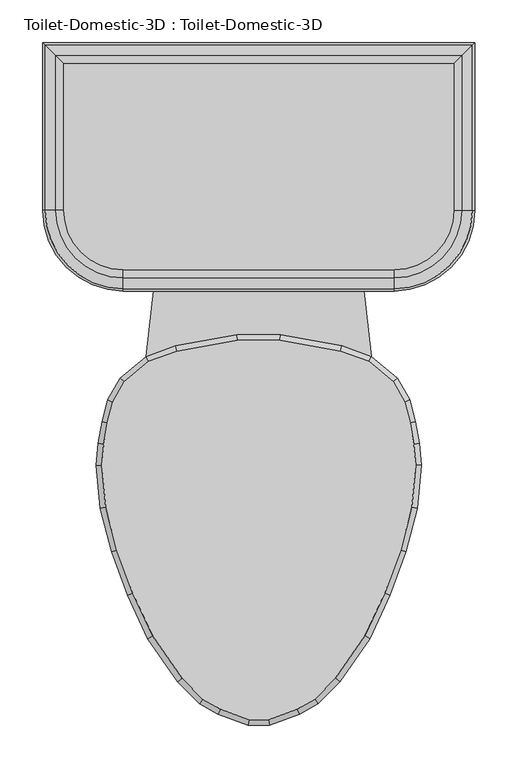
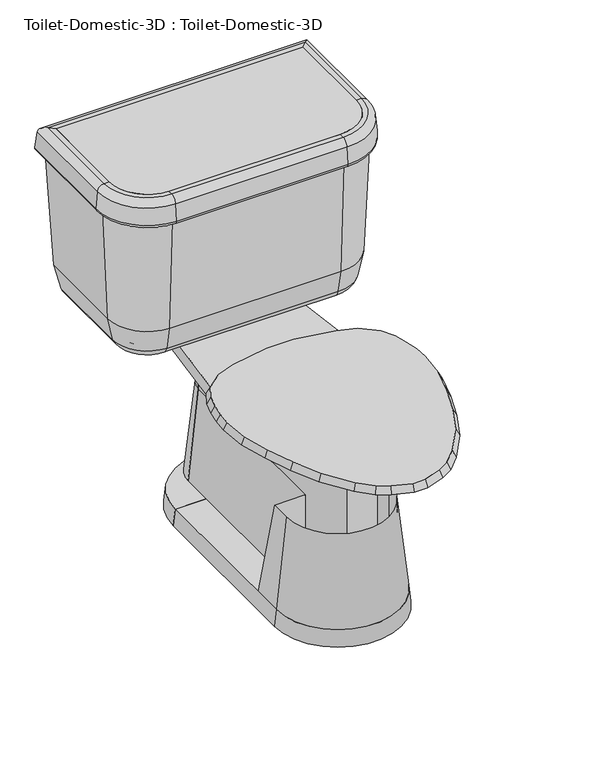
"""IFC4 building model written with IfcOpenShell, lengths in millimetres: flow terminal geometry, Toilet-Domestic-3D : Toilet-Domestic-3D."""

from ifc_helpers import new_model, si_unit, point, frame, frame_2d, origin, place, context, project, spatial, polyline, circle_curve, ellipse_curve, trimmed, segment, composite_curve, outline, extrude, faceted_brep, source, transform, mapped, element, save
from ifc_brep_helpers import plane_surface, cylinder_surface, revolved_surface, advanced_brep


def toilet_domestic_3d_toilet_domestic_3d_f7549cf7(model_context):
    return source(origin(), model_context, "Body", "SolidModel", [
        advanced_brep(
        [(-117.7636364, 285.75, 0.0), (-38.1, 285.75, 0.0), (-38.1, 285.75, 31.75), (-114.3, 285.75, 31.75), (117.7636364, 285.75, 0.0), (114.3, 285.75, 31.75), (38.1, 285.75, 31.75), (38.1, 285.75, 0.0)],
        [
            (0, 1),
            (1, 2),
            (2, 3),
            (3, 0),
            (4, 5),
            (5, 6),
            (6, 7),
            (7, 4),
            (7, 1, circle_curve(frame((0.0, 285.75, 0.0), z_axis=(0.0, 0.0, 1.0), x_axis=(-1.0, 0.0, 0.0)), 38.1)),
            (0, 4, circle_curve(frame((0.0, 285.75, 0.0), z_axis=(0.0, 0.0, -1.0), x_axis=(-1.0, 0.0, 0.0)), 117.7636364)),
            (6, 2, circle_curve(frame((0.0, 285.75, 31.75), z_axis=(0.0, 0.0, 1.0), x_axis=(-1.0, 0.0, 0.0)), 38.1)),
            (5, 3, circle_curve(frame((0.0, 285.75, 31.75), z_axis=(0.0, 0.0, 1.0), x_axis=(-1.0, 0.0, 0.0)), 114.3)),
        ],
        [
            plane_surface(frame((0.0, 285.75, -304.8), z_axis=(0.0, -1.0, 0.0), x_axis=(-1.0, 0.0, 0.0))),
            plane_surface(frame((0.0, 285.75, -304.8), z_axis=(0.0, -1.0, 0.0), x_axis=(1.0, 0.0, 0.0))),
            plane_surface(frame((0.0, 285.75, 0.0), z_axis=(0.0, 0.0, -1.0), x_axis=(-1.0, 0.0, 0.0))),
            revolved_surface(polyline([(-38.1, 285.75, 0.0), (-38.1, 285.75, 31.75)]), (0.0, 285.75, -304.8), (0.0, 0.0, -1.0)),
            plane_surface(frame((0.0, 285.75, 31.75), z_axis=(0.0, 0.0, 1.0), x_axis=(-1.0, 0.0, 0.0))),
            revolved_surface(polyline([(-114.3, 285.75, 31.75), (-117.7636364, 285.75, 0.0)]), (0.0, 285.75, -304.8), (0.0, 0.0, -1.0)),
        ],
        [
            (0, [[1, 2, 3, 4]]),
            (1, [[5, 6, 7, 8]]),
            (2, [[9, -1, 10, -8]]),
            (3, [[11, -2, -9, -7]]),
            (4, [[12, -3, -11, -6]]),
            (5, [[-10, -4, -12, -5]]),
        ],
    ),
        advanced_brep(
        [(-38.1, 342.9, 206.375), (-57.15, 342.9, 31.75), (-38.1, 342.9, 31.75), (38.1, 342.9, 206.375), (38.1, 342.9, 31.75), (57.15, 342.9, 31.75)],
        [
            (0, 1),
            (1, 2),
            (2, 0),
            (3, 4),
            (4, 5),
            (5, 3),
            (5, 1, circle_curve(frame((0.0, 342.9, 31.75), z_axis=(0.0, 0.0, 1.0), x_axis=(-1.0, 0.0, 0.0)), 57.15)),
            (0, 3, circle_curve(frame((0.0, 342.9, 206.375), z_axis=(0.0, 0.0, -1.0), x_axis=(-1.0, 0.0, 0.0)), 38.1)),
            (4, 2, circle_curve(frame((0.0, 342.9, 31.75), z_axis=(0.0, 0.0, 1.0), x_axis=(-1.0, 0.0, 0.0)), 38.1)),
        ],
        [
            plane_surface(frame((0.0, 342.9, 31.75), z_axis=(0.0, -1.0, 0.0), x_axis=(-1.0, 0.0, 0.0))),
            plane_surface(frame((0.0, 342.9, 31.75), z_axis=(0.0, -1.0, 0.0), x_axis=(1.0, 0.0, 0.0))),
            revolved_surface(polyline([(-38.1, 342.9, 206.375), (-57.15, 342.9, 31.75)]), (0.0, 342.9, 31.75), (0.0, 0.0, -1.0)),
            plane_surface(frame((0.0, 342.9, 31.75), z_axis=(0.0, 0.0, -1.0), x_axis=(-1.0, 0.0, 0.0))),
            revolved_surface(polyline([(-38.1, 342.9, 31.75), (-38.1, 342.9, 206.375)]), (0.0, 342.9, 31.75), (0.0, 0.0, -1.0)),
        ],
        [
            (0, [[1, 2, 3]]),
            (1, [[4, 5, 6]]),
            (2, [[7, -1, 8, -6]]),
            (3, [[9, -2, -7, -5]]),
            (4, [[-8, -3, -9, -4]]),
        ],
    ),
        faceted_brep([(-157.6293435, 97.472128, 400.05), (-171.060664, 73.773864, 400.05), (-177.5851102, 49.4242991, 400.05), (-181.9845715, 24.4737144, 400.05), (-184.125744, 0.0, 400.05), (-179.7950716, -49.4998127, 400.05), (-166.347, -99.688699, 400.05), (-148.0469602, -149.9676451, 400.05), (-124.7045808, -200.0255393, 400.05), (-90.0971582, -249.9125941, 400.05), (-65.691017, -274.3187354, 400.05), (-44.8990862, -286.3229622, 400.05), (-11.5803237, -298.45, 400.05), (11.5803237, -298.45, 400.05), (44.8990862, -286.3229622, 400.05), (65.691017, -274.3187354, 400.05), (90.0971582, -249.9125941, 400.05), (124.7045808, -200.0255393, 400.05), (148.0469602, -149.9676451, 400.05), (166.347, -99.688699, 400.05), (179.7950716, -49.4998127, 400.05), (184.125744, 0.0, 400.05), (181.9845715, 24.4737144, 400.05), (177.5851102, 49.4242991, 400.05), (171.060664, 73.773864, 400.05), (157.6293435, 97.472128, 400.05), (129.0942628, 121.4159037, 400.05), (95.7755003, 133.5429415, 400.05), (24.844447, 146.05, 400.05), (-24.844447, 146.05, 400.05), (-95.7755003, 133.5429415, 400.05), (-129.0942628, 121.4159037, 400.05), (-162.5887836, 101.6, 387.2181453), (-132.3182423, 127.0, 387.2181453), (-97.4252791, 139.7, 387.2181453), (-25.4, 152.4, 387.2181453), (25.4, 152.4, 387.2181453), (97.4252791, 139.7, 387.2181453), (132.3182423, 127.0, 387.2181453), (162.5887836, 101.6, 387.2181453), (176.9845865, 76.2, 387.2181453), (183.790496, 50.8, 387.2181453), (188.2862441, 25.3033453, 387.2181453), (190.5, 0.0, 387.2181453), (186.0724883, -50.6066907, 387.2181453), (172.4088722, -101.6, 387.2181453), (153.9191843, -152.4, 387.2181453), (130.2307553, -203.2, 387.2181453), (94.9900085, -254.0, 387.2181453), (69.5900085, -279.4, 387.2181453), (47.5929632, -292.1, 387.2181453), (12.7, -304.8, 387.2181453), (-12.7, -304.8, 387.2181453), (-47.5929632, -292.1, 387.2181453), (-69.5900085, -279.4, 387.2181453), (-94.9900085, -254.0, 387.2181453), (-130.2307553, -203.2, 387.2181453), (-153.9191843, -152.4, 387.2181453), (-172.4088722, -101.6, 387.2181453), (-186.0724883, -50.6066907, 387.2181453), (-190.5, 0.0, 387.2181453), (-188.2862441, 25.3033453, 387.2181453), (-183.790496, 50.8, 387.2181453), (-176.9845865, 76.2, 387.2181453)], [[[0, 1, 2, 3, 4, 5, 6, 7, 8, 9, 10, 11, 12, 13, 14, 15, 16, 17, 18, 19, 20, 21, 22, 23, 24, 25, 26, 27, 28, 29, 30, 31]], [[32, 33, 34, 35, 36, 37, 38, 39, 40, 41, 42, 43, 44, 45, 46, 47, 48, 49, 50, 51, 52, 53, 54, 55, 56, 57, 58, 59, 60, 61, 62, 63]], [[32, 63, 1, 0]], [[63, 62, 2, 1]], [[62, 61, 3, 2]], [[61, 60, 4, 3]], [[60, 59, 5, 4]], [[59, 58, 6, 5]], [[58, 57, 7, 6]], [[57, 56, 8, 7]], [[56, 55, 9, 8]], [[55, 54, 10, 9]], [[54, 53, 11, 10]], [[53, 52, 12, 11]], [[52, 51, 13, 12]], [[51, 50, 14, 13]], [[50, 49, 15, 14]], [[49, 48, 16, 15]], [[48, 47, 17, 16]], [[47, 46, 18, 17]], [[46, 45, 19, 18]], [[45, 44, 20, 19]], [[44, 43, 21, 20]], [[43, 42, 22, 21]], [[42, 41, 23, 22]], [[41, 40, 24, 23]], [[40, 39, 25, 24]], [[39, 38, 26, 25]], [[38, 37, 27, 26]], [[37, 36, 28, 27]], [[36, 35, 29, 28]], [[35, 34, 30, 29]], [[34, 33, 31, 30]], [[33, 32, 0, 31]]]),
        extrude(outline(composite_curve([segment(polyline([(228.5868869, 469.8868869), (228.5868869, 298.45)]), True, "CONTINUOUS"), segment(trimmed(circle_curve(frame_2d((158.75, 298.45)), 69.8368869), [point((228.5868869, 298.45))], [point((158.75, 228.6131131))], False, "CARTESIAN"), True, "CONTINUOUS"), segment(polyline([(158.75, 228.6131131), (-158.75, 228.6131131)]), True, "CONTINUOUS"), segment(trimmed(circle_curve(frame_2d((-158.75, 298.45)), 69.8368869), [point((-158.75, 228.6131131))], [point((-228.5868869, 298.45))], False, "CARTESIAN"), True, "CONTINUOUS"), segment(polyline([(-228.5868869, 298.45), (-228.5868869, 469.8868869), (228.5868869, 469.8868869)]), True, "CONTINUOUS")], self_intersect=False)), frame((0.0, 0.0, 654.05), z_axis=(0.0, 0.0, 1.0), x_axis=(1.0, 0.0, 0.0)), (0.0, 0.0, 1.0), 50.8),
        extrude(outline(composite_curve([segment(trimmed(circle_curve(frame_2d((0.0, 342.9)), 38.1), [point((-38.1, 342.9))], [point((38.1, 342.9))], False, "CARTESIAN"), True, "CONTINUOUS"), segment(polyline([(38.1, 342.9), (-38.1, 342.9)]), True, "CONTINUOUS")], self_intersect=False)), frame((0.0, 0.0, 206.375), z_axis=(0.0, 0.0, 1.0), x_axis=(1.0, 0.0, 0.0)), (0.0, 0.0, 1.0), 130.175),
        advanced_brep(
        [(177.8, 419.1, 387.2181453), (177.8, 419.1, 374.65), (177.8, 298.45, 374.65), (177.8, 298.45, 387.2181453), (192.8020829, 434.1020829, 387.2181453), (192.8020829, 298.45, 387.2181453), (211.4650931, 452.7650931, 402.4478636), (211.4650931, 298.45, 402.4478636), (218.7732506, 460.0732506, 438.15), (218.7732506, 298.45, 438.15), (228.5868869, 469.8868869, 654.05), (228.5868869, 298.45, 654.05), (228.5868869, 469.8868869, 704.85), (228.5868869, 298.45, 704.85), (237.91817, 479.21817, 704.85), (237.91817, 298.45, 704.85), (250.5698426, 491.8698426, 693.2568779), (250.5698426, 298.45, 693.2568779), (253.3960274, 494.6960274, 660.953439), (253.3960274, 298.45, 660.953439), (247.070191, 488.370191, 654.05), (247.070191, 298.45, 654.05), (241.3, 482.6, 654.05), (241.3, 298.45, 654.05), (231.4863636, 472.7863636, 438.15), (231.4863636, 298.45, 438.15), (222.3416824, 463.6416824, 393.4759963), (222.3416824, 298.45, 393.4759963), (197.8071664, 439.1071664, 374.65), (197.8071664, 298.45, 374.65), (158.75, 279.4, 387.2181453), (158.75, 279.4, 374.65), (158.75, 264.3979171, 387.2181453), (158.75, 245.7349069, 402.4478636), (158.75, 238.4267494, 438.15), (158.75, 228.6131131, 654.05), (158.75, 228.6131131, 704.85), (158.75, 219.28183, 704.85), (158.75, 206.6301574, 693.2568779), (158.75, 203.8039726, 660.953439), (158.75, 210.129809, 654.05), (158.75, 215.9, 654.05), (158.75, 225.7136364, 438.15), (158.75, 234.8583176, 393.4759963), (158.75, 259.3928336, 374.65), (-158.75, 279.4, 374.65), (-158.75, 279.4, 387.2181453), (-158.75, 264.3979171, 387.2181453), (-158.75, 245.7349069, 402.4478636), (-158.75, 238.4267494, 438.15), (-158.75, 228.6131131, 654.05), (-158.75, 228.6131131, 704.85), (-158.75, 219.28183, 704.85), (-158.75, 206.6301574, 693.2568779), (-158.75, 203.8039726, 660.953439), (-158.75, 210.129809, 654.05), (-158.75, 215.9, 654.05), (-158.75, 225.7136364, 438.15), (-158.75, 234.8583176, 393.4759963), (-158.75, 259.3928336, 374.65), (-177.8, 298.45, 387.2181453), (-177.8, 298.45, 374.65), (-192.8020829, 298.45, 387.2181453), (-211.4650931, 298.45, 402.4478636), (-218.7732506, 298.45, 438.15), (-228.5868869, 298.45, 654.05), (-228.5868869, 298.45, 704.85), (-237.91817, 298.45, 704.85), (-250.5698426, 298.45, 693.2568779), (-253.3960274, 298.45, 660.953439), (-247.070191, 298.45, 654.05), (-241.3, 298.45, 654.05), (-231.4863636, 298.45, 438.15), (-222.3416824, 298.45, 393.4759963), (-197.8071664, 298.45, 374.65), (-177.8, 419.1, 374.65), (-177.8, 419.1, 387.2181453), (-192.8020829, 434.1020829, 387.2181453), (-211.4650931, 452.7650931, 402.4478636), (-218.7732506, 460.0732506, 438.15), (-228.5868869, 469.8868869, 654.05), (-228.5868869, 469.8868869, 704.85), (-237.91817, 479.21817, 704.85), (-250.5698426, 491.8698426, 693.2568779), (-253.3960274, 494.6960274, 660.953439), (-247.070191, 488.370191, 654.05), (-241.3, 482.6, 654.05), (-231.4863636, 472.7863636, 438.15), (-222.3416824, 463.6416824, 393.4759963), (-197.8071664, 439.1071664, 374.65)],
        [
            (0, 1),
            (1, 2),
            (2, 3),
            (3, 0),
            (4, 0),
            (3, 5),
            (5, 4),
            (6, 4, ellipse_curve(frame((192.8020829, 434.1020829, 406.2681453), z_axis=(-0.7071067811865451, 0.7071067811865498, 0.0), x_axis=(-0.7071067811865497, -0.7071067811865452, 0.0)), 26.9407684, 19.05)),
            (5, 7, circle_curve(frame((192.8020829, 298.45, 406.2681453), z_axis=(0.0, -1.0, 0.0), x_axis=(1.0, 0.0, 0.0)), 19.05)),
            (7, 6),
            (8, 6),
            (7, 9),
            (9, 8),
            (10, 8),
            (9, 11),
            (11, 10),
            (12, 10),
            (11, 13),
            (13, 12),
            (14, 12),
            (13, 15),
            (15, 14),
            (16, 14, ellipse_curve(frame((237.91817, 479.21817, 692.15), z_axis=(0.7071067811865451, -0.7071067811865498, 0.0), x_axis=(0.7071067811865497, 0.7071067811865452, 0.0)), 17.9605122, 12.7)),
            (15, 17, circle_curve(frame((237.91817, 298.45, 692.15), z_axis=(0.0, 1.0, 0.0), x_axis=(1.0, 0.0, 0.0)), 12.7)),
            (17, 16),
            (18, 16),
            (17, 19),
            (19, 18),
            (20, 18, ellipse_curve(frame((247.070191, 488.370191, 660.4), z_axis=(0.7071067811865451, -0.7071067811865498, 0.0), x_axis=(0.7071067811865497, 0.7071067811865452, 0.0)), 8.9802561, 6.35)),
            (19, 21, circle_curve(frame((247.070191, 298.45, 660.4), z_axis=(0.0, 1.0, 0.0), x_axis=(1.0, 0.0, 0.0)), 6.35)),
            (21, 20),
            (22, 20),
            (21, 23),
            (23, 22),
            (24, 22),
            (23, 25),
            (25, 24),
            (26, 24),
            (25, 27),
            (27, 26),
            (28, 26, ellipse_curve(frame((197.8071664, 439.1071664, 400.05), z_axis=(0.7071067811865451, -0.7071067811865498, 0.0), x_axis=(0.7071067811865497, 0.7071067811865452, 0.0)), 35.9210245, 25.4)),
            (27, 29, circle_curve(frame((197.8071664, 298.45, 400.05), z_axis=(0.0, 1.0, 0.0), x_axis=(1.0, 0.0, 0.0)), 25.4)),
            (29, 28),
            (1, 28),
            (29, 2),
            (30, 3, circle_curve(frame((158.75, 298.45, 387.2181453), z_axis=(0.0, 0.0, 1.0), x_axis=(1.0, 0.0, 0.0)), 19.05)),
            (2, 31, circle_curve(frame((158.75, 298.45, 374.65), z_axis=(0.0, 0.0, -1.0), x_axis=(1.0, 0.0, 0.0)), 19.05)),
            (31, 30),
            (32, 5, circle_curve(frame((158.75, 298.45, 387.2181453), z_axis=(0.0, 0.0, 1.0), x_axis=(1.0, 0.0, 0.0)), 34.0520829)),
            (30, 32),
            (33, 7, circle_curve(frame((158.75, 298.45, 402.4478636), z_axis=(0.0, 0.0, 1.0), x_axis=(1.0, 0.0, 0.0)), 52.7150931)),
            (32, 33, circle_curve(frame((158.75, 264.3979171, 406.2681453), z_axis=(-1.0, 0.0, 0.0), x_axis=(0.0, -1.0, 0.0)), 19.05)),
            (34, 9, circle_curve(frame((158.75, 298.45, 438.15), z_axis=(0.0, 0.0, 1.0), x_axis=(1.0, 0.0, 0.0)), 60.0232506)),
            (33, 34),
            (35, 11, circle_curve(frame((158.75, 298.45, 654.05), z_axis=(0.0, 0.0, 1.0), x_axis=(1.0, 0.0, 0.0)), 69.8368869)),
            (34, 35),
            (36, 13, circle_curve(frame((158.75, 298.45, 704.85), z_axis=(0.0, 0.0, 1.0), x_axis=(1.0, 0.0, 0.0)), 69.8368869)),
            (35, 36),
            (37, 15, circle_curve(frame((158.75, 298.45, 704.85), z_axis=(0.0, 0.0, 1.0), x_axis=(1.0, 0.0, 0.0)), 79.16817)),
            (36, 37),
            (38, 17, circle_curve(frame((158.75, 298.45, 693.2568779), z_axis=(0.0, 0.0, 1.0), x_axis=(1.0, 0.0, 0.0)), 91.8198426)),
            (37, 38, circle_curve(frame((158.75, 219.28183, 692.15), z_axis=(1.0, 0.0, 0.0), x_axis=(0.0, -1.0, 0.0)), 12.7)),
            (39, 19, circle_curve(frame((158.75, 298.45, 660.953439), z_axis=(0.0, 0.0, 1.0), x_axis=(1.0, 0.0, 0.0)), 94.6460274)),
            (38, 39),
            (40, 21, circle_curve(frame((158.75, 298.45, 654.05), z_axis=(0.0, 0.0, 1.0), x_axis=(1.0, 0.0, 0.0)), 88.320191)),
            (39, 40, circle_curve(frame((158.75, 210.129809, 660.4), z_axis=(1.0, 0.0, 0.0), x_axis=(0.0, -1.0, 0.0)), 6.35)),
            (41, 23, circle_curve(frame((158.75, 298.45, 654.05), z_axis=(0.0, 0.0, 1.0), x_axis=(1.0, 0.0, 0.0)), 82.55)),
            (40, 41),
            (42, 25, circle_curve(frame((158.75, 298.45, 438.15), z_axis=(0.0, 0.0, 1.0), x_axis=(1.0, 0.0, 0.0)), 72.7363636)),
            (41, 42),
            (43, 27, circle_curve(frame((158.75, 298.45, 393.4759963), z_axis=(0.0, 0.0, 1.0), x_axis=(1.0, 0.0, 0.0)), 63.5916824)),
            (42, 43),
            (44, 29, circle_curve(frame((158.75, 298.45, 374.65), z_axis=(0.0, 0.0, 1.0), x_axis=(1.0, 0.0, 0.0)), 39.0571664)),
            (43, 44, circle_curve(frame((158.75, 259.3928336, 400.05), z_axis=(1.0, 0.0, 0.0), x_axis=(0.0, -1.0, 0.0)), 25.4)),
            (44, 31),
            (31, 45),
            (45, 46),
            (46, 30),
            (46, 47),
            (47, 32),
            (47, 48, circle_curve(frame((-158.75, 264.3979171, 406.2681453), z_axis=(-1.0, 0.0, 0.0), x_axis=(0.0, -1.0, 0.0)), 19.05)),
            (48, 33),
            (48, 49),
            (49, 34),
            (49, 50),
            (50, 35),
            (50, 51),
            (51, 36),
            (51, 52),
            (52, 37),
            (52, 53, circle_curve(frame((-158.75, 219.28183, 692.15), z_axis=(1.0, 0.0, 0.0), x_axis=(0.0, -1.0, 0.0)), 12.7)),
            (53, 38),
            (53, 54),
            (54, 39),
            (54, 55, circle_curve(frame((-158.75, 210.129809, 660.4), z_axis=(1.0, 0.0, 0.0), x_axis=(0.0, -1.0, 0.0)), 6.35)),
            (55, 40),
            (55, 56),
            (56, 41),
            (56, 57),
            (57, 42),
            (57, 58),
            (58, 43),
            (58, 59, circle_curve(frame((-158.75, 259.3928336, 400.05), z_axis=(1.0, 0.0, 0.0), x_axis=(0.0, -1.0, 0.0)), 25.4)),
            (59, 44),
            (59, 45),
            (60, 46, circle_curve(frame((-158.75, 298.45, 387.2181453), z_axis=(0.0, 0.0, 1.0), x_axis=(0.0, -1.0, 0.0)), 19.05)),
            (45, 61, circle_curve(frame((-158.75, 298.45, 374.65), z_axis=(0.0, 0.0, -1.0), x_axis=(0.0, -1.0, 0.0)), 19.05)),
            (61, 60),
            (62, 47, circle_curve(frame((-158.75, 298.45, 387.2181453), z_axis=(0.0, 0.0, 1.0), x_axis=(0.0, -1.0, 0.0)), 34.0520829)),
            (60, 62),
            (63, 48, circle_curve(frame((-158.75, 298.45, 402.4478636), z_axis=(0.0, 0.0, 1.0), x_axis=(0.0, -1.0, 0.0)), 52.7150931)),
            (62, 63, circle_curve(frame((-192.8020829, 298.45, 406.2681453), z_axis=(0.0, 1.0, 0.0), x_axis=(-1.0, 0.0, 0.0)), 19.05)),
            (64, 49, circle_curve(frame((-158.75, 298.45, 438.15), z_axis=(0.0, 0.0, 1.0), x_axis=(0.0, -1.0, 0.0)), 60.0232506)),
            (63, 64),
            (65, 50, circle_curve(frame((-158.75, 298.45, 654.05), z_axis=(0.0, 0.0, 1.0), x_axis=(0.0, -1.0, 0.0)), 69.8368869)),
            (64, 65),
            (66, 51, circle_curve(frame((-158.75, 298.45, 704.85), z_axis=(0.0, 0.0, 1.0), x_axis=(0.0, -1.0, 0.0)), 69.8368869)),
            (65, 66),
            (67, 52, circle_curve(frame((-158.75, 298.45, 704.85), z_axis=(0.0, 0.0, 1.0), x_axis=(0.0, -1.0, 0.0)), 79.16817)),
            (66, 67),
            (68, 53, circle_curve(frame((-158.75, 298.45, 693.2568779), z_axis=(0.0, 0.0, 1.0), x_axis=(0.0, -1.0, 0.0)), 91.8198426)),
            (67, 68, circle_curve(frame((-237.91817, 298.45, 692.15), z_axis=(0.0, -1.0, 0.0), x_axis=(-1.0, 0.0, 0.0)), 12.7)),
            (69, 54, circle_curve(frame((-158.75, 298.45, 660.953439), z_axis=(0.0, 0.0, 1.0), x_axis=(0.0, -1.0, 0.0)), 94.6460274)),
            (68, 69),
            (70, 55, circle_curve(frame((-158.75, 298.45, 654.05), z_axis=(0.0, 0.0, 1.0), x_axis=(0.0, -1.0, 0.0)), 88.320191)),
            (69, 70, circle_curve(frame((-247.070191, 298.45, 660.4), z_axis=(0.0, -1.0, 0.0), x_axis=(-1.0, 0.0, 0.0)), 6.35)),
            (71, 56, circle_curve(frame((-158.75, 298.45, 654.05), z_axis=(0.0, 0.0, 1.0), x_axis=(0.0, -1.0, 0.0)), 82.55)),
            (70, 71),
            (72, 57, circle_curve(frame((-158.75, 298.45, 438.15), z_axis=(0.0, 0.0, 1.0), x_axis=(0.0, -1.0, 0.0)), 72.7363636)),
            (71, 72),
            (73, 58, circle_curve(frame((-158.75, 298.45, 393.4759963), z_axis=(0.0, 0.0, 1.0), x_axis=(0.0, -1.0, 0.0)), 63.5916824)),
            (72, 73),
            (74, 59, circle_curve(frame((-158.75, 298.45, 374.65), z_axis=(0.0, 0.0, 1.0), x_axis=(0.0, -1.0, 0.0)), 39.0571664)),
            (73, 74, circle_curve(frame((-197.8071664, 298.45, 400.05), z_axis=(0.0, -1.0, 0.0), x_axis=(-1.0, 0.0, 0.0)), 25.4)),
            (74, 61),
            (61, 75),
            (75, 76),
            (76, 60),
            (76, 77),
            (77, 62),
            (77, 78, ellipse_curve(frame((-192.8020829, 434.1020829, 406.2681453), z_axis=(0.7071067811865498, 0.7071067811865451, 0.0), x_axis=(-0.7071067811865451, 0.70710678118655, 0.0)), 26.9407684, 19.05)),
            (78, 63),
            (78, 79),
            (79, 64),
            (79, 80),
            (80, 65),
            (80, 81),
            (81, 66),
            (81, 82),
            (82, 67),
            (82, 83, ellipse_curve(frame((-237.91817, 479.21817, 692.15), z_axis=(-0.7071067811865498, -0.7071067811865451, 0.0), x_axis=(0.7071067811865451, -0.70710678118655, 0.0)), 17.9605122, 12.7)),
            (83, 68),
            (83, 84),
            (84, 69),
            (84, 85, ellipse_curve(frame((-247.070191, 488.370191, 660.4), z_axis=(-0.7071067811865498, -0.7071067811865451, 0.0), x_axis=(0.7071067811865451, -0.70710678118655, 0.0)), 8.9802561, 6.35)),
            (85, 70),
            (85, 86),
            (86, 71),
            (86, 87),
            (87, 72),
            (87, 88),
            (88, 73),
            (88, 89, ellipse_curve(frame((-197.8071664, 439.1071664, 400.05), z_axis=(-0.7071067811865498, -0.7071067811865451, 0.0), x_axis=(0.7071067811865451, -0.70710678118655, 0.0)), 35.9210245, 25.4)),
            (89, 74),
            (89, 75),
            (75, 1),
            (0, 76),
            (4, 77),
            (6, 78),
            (8, 79),
            (10, 80),
            (12, 81),
            (14, 82),
            (16, 83),
            (18, 84),
            (20, 85),
            (22, 86),
            (24, 87),
            (26, 88),
            (28, 89),
        ],
        [
            plane_surface(frame((177.8, 419.1, 374.65), z_axis=(-1.0, 0.0, 0.0), x_axis=(0.0, -1.0, 0.0))),
            plane_surface(frame((177.8, 419.1, 387.2181453), z_axis=(0.0, 0.0, 1.0), x_axis=(0.0, -1.0, 0.0))),
            revolved_surface(polyline([(211.8520829, 298.45, 406.2681453), (211.8520829, 453.1520829260162, 406.2681453)]), (192.8020829, 419.1, 406.2681453), (0.0, -1.0, 0.0)),
            plane_surface(frame((211.4650931, 452.7650931, 402.4478636), z_axis=(-0.9796855721787505, 0.0, 0.2005397209153197), x_axis=(0.0, -1.0, 0.0))),
            plane_surface(frame((218.7732506, 460.0732506, 438.15), z_axis=(-0.9989685402102995, 0.0, 0.045407660918654086), x_axis=(0.0, -1.0, 0.0))),
            plane_surface(frame((228.5868869, 469.8868869, 654.05), z_axis=(-1.0, 0.0, 0.0), x_axis=(0.0, -1.0, 0.0))),
            plane_surface(frame((228.5868869, 469.8868869, 704.85), z_axis=(0.0, 0.0, 1.0), x_axis=(0.0, -1.0, 0.0))),
            cylinder_surface(frame((237.91817, 419.1, 692.15), z_axis=(0.0, 1.0, 0.0), x_axis=(1.0, 0.0, 0.0)), 12.7),
            plane_surface(frame((250.5698426, 491.8698426, 693.2568779), z_axis=(0.9961946980917452, 0.0, 0.08715574274766269), x_axis=(0.0, -1.0, 0.0))),
            cylinder_surface(frame((247.070191, 419.1, 660.4), z_axis=(0.0, 1.0, 0.0), x_axis=(1.0, 0.0, 0.0)), 6.35),
            plane_surface(frame((247.070191, 488.370191, 654.05), z_axis=(0.0, 0.0, -1.0), x_axis=(0.0, -1.0, 0.0))),
            plane_surface(frame((241.3, 482.6, 654.05), z_axis=(0.9989685402102993, 0.0, -0.04540766091865594), x_axis=(0.0, -1.0, 0.0))),
            plane_surface(frame((231.4863636, 472.7863636, 438.15), z_axis=(0.9796855721787489, 0.0, -0.20053972091532798), x_axis=(0.0, -1.0, 0.0))),
            cylinder_surface(frame((197.8071664, 419.1, 400.05), z_axis=(0.0, 1.0, 0.0), x_axis=(1.0, 0.0, 0.0)), 25.4),
            plane_surface(frame((197.8071664, 439.1071664, 374.65), z_axis=(0.0, 0.0, -1.0), x_axis=(0.0, -1.0, 0.0))),
            revolved_surface(polyline([(177.8, 298.45, 374.65), (177.8, 298.45, 387.2181453)]), (158.75, 298.45, 0.0), (0.0, 0.0, -1.0)),
            plane_surface(frame((158.75, 298.45, 387.2181453), z_axis=(0.0, 0.0, 1.0), x_axis=(1.0, 0.0, 0.0))),
            revolved_surface(trimmed(ellipse_curve(frame((192.8020829, 298.45, 406.2681453), z_axis=(0.0, -1.0, 0.0), x_axis=(1.0, 0.0, 0.0)), 19.05, 19.05), [point((192.8020829, 298.45, 387.2181453))], [point((211.4650931, 298.45, 402.4478636))], True, "CARTESIAN"), (158.75, 298.45, 0.0), (0.0, 0.0, -1.0)),
            revolved_surface(polyline([(211.4650931, 298.45, 402.4478636), (218.7732506, 298.45, 438.15)]), (158.75, 298.45, 0.0), (0.0, 0.0, -1.0)),
            revolved_surface(polyline([(218.7732506, 298.45, 438.15), (228.5868869, 298.45, 654.05)]), (158.75, 298.45, 0.0), (0.0, 0.0, -1.0)),
            revolved_surface(polyline([(228.5868869, 298.45, 654.05), (228.5868869, 298.45, 704.85)]), (158.75, 298.45, 0.0), (0.0, 0.0, -1.0)),
            plane_surface(frame((158.75, 298.45, 704.85), z_axis=(0.0, 0.0, 1.0), x_axis=(1.0, 0.0, 0.0))),
            revolved_surface(trimmed(ellipse_curve(frame((237.91817, 298.45, 692.15), z_axis=(0.0, 1.0, 0.0), x_axis=(1.0, 0.0, 0.0)), 12.7, 12.7), [point((237.91817, 298.45, 704.85))], [point((250.5698426, 298.45, 693.2568779))], True, "CARTESIAN"), (158.75, 298.45, 0.0), (0.0, 0.0, -1.0)),
            revolved_surface(polyline([(250.5698426, 298.45, 693.2568779), (253.3960274, 298.45, 660.953439)]), (158.75, 298.45, 0.0), (0.0, 0.0, -1.0)),
            revolved_surface(trimmed(ellipse_curve(frame((247.070191, 298.45, 660.4), z_axis=(0.0, 1.0, 0.0), x_axis=(1.0, 0.0, 0.0)), 6.35, 6.35), [point((253.3960274, 298.45, 660.953439))], [point((247.070191, 298.45, 654.05))], True, "CARTESIAN"), (158.75, 298.45, 0.0), (0.0, 0.0, -1.0)),
            plane_surface(frame((158.75, 298.45, 654.05), z_axis=(0.0, 0.0, -1.0), x_axis=(1.0, 0.0, 0.0))),
            revolved_surface(polyline([(241.3, 298.45, 654.05), (231.4863636, 298.45, 438.15)]), (158.75, 298.45, 0.0), (0.0, 0.0, -1.0)),
            revolved_surface(polyline([(231.4863636, 298.45, 438.15), (222.3416824, 298.45, 393.4759963)]), (158.75, 298.45, 0.0), (0.0, 0.0, -1.0)),
            revolved_surface(trimmed(ellipse_curve(frame((197.8071664, 298.45, 400.05), z_axis=(0.0, 1.0, 0.0), x_axis=(1.0, 0.0, 0.0)), 25.4, 25.4), [point((222.3416824, 298.45, 393.4759963))], [point((197.8071664, 298.45, 374.65))], True, "CARTESIAN"), (158.75, 298.45, 0.0), (0.0, 0.0, -1.0)),
            plane_surface(frame((158.75, 298.45, 374.65), z_axis=(0.0, 0.0, -1.0), x_axis=(1.0, 0.0, 0.0))),
            plane_surface(frame((158.75, 279.4, 374.65), z_axis=(0.0, 1.0, 0.0), x_axis=(-1.0, 0.0, 0.0))),
            plane_surface(frame((158.75, 279.4, 387.2181453), z_axis=(0.0, 0.0, 1.0), x_axis=(-1.0, 0.0, 0.0))),
            revolved_surface(polyline([(-158.75, 245.34791709999996, 406.2681453), (158.75, 245.34791709999996, 406.2681453)]), (158.75, 264.3979171, 406.2681453), (-1.0, 0.0, 0.0)),
            plane_surface(frame((158.75, 245.7349069, 402.4478636), z_axis=(0.0, 0.9796855721787505, 0.2005397209153197), x_axis=(-1.0, 0.0, 0.0))),
            plane_surface(frame((158.75, 238.4267494, 438.15), z_axis=(0.0, 0.9989685402102995, 0.045407660918654086), x_axis=(-1.0, 0.0, 0.0))),
            plane_surface(frame((158.75, 228.6131131, 654.05), z_axis=(0.0, 1.0, 0.0), x_axis=(-1.0, 0.0, 0.0))),
            plane_surface(frame((158.75, 228.6131131, 704.85), z_axis=(0.0, 0.0, 1.0), x_axis=(-1.0, 0.0, 0.0))),
            cylinder_surface(frame((158.75, 219.28183, 692.15), z_axis=(1.0, 0.0, 0.0), x_axis=(0.0, -1.0, 0.0)), 12.7),
            plane_surface(frame((158.75, 206.6301574, 693.2568779), z_axis=(0.0, -0.9961946980917452, 0.08715574274766269), x_axis=(-1.0, 0.0, 0.0))),
            cylinder_surface(frame((158.75, 210.129809, 660.4), z_axis=(1.0, 0.0, 0.0), x_axis=(0.0, -1.0, 0.0)), 6.35),
            plane_surface(frame((158.75, 210.129809, 654.05), z_axis=(0.0, 0.0, -1.0), x_axis=(-1.0, 0.0, 0.0))),
            plane_surface(frame((158.75, 215.9, 654.05), z_axis=(0.0, -0.9989685402102993, -0.04540766091865594), x_axis=(-1.0, 0.0, 0.0))),
            plane_surface(frame((158.75, 225.7136364, 438.15), z_axis=(0.0, -0.9796855721787489, -0.20053972091532798), x_axis=(-1.0, 0.0, 0.0))),
            cylinder_surface(frame((158.75, 259.3928336, 400.05), z_axis=(1.0, 0.0, 0.0), x_axis=(0.0, -1.0, 0.0)), 25.4),
            plane_surface(frame((158.75, 259.3928336, 374.65), z_axis=(0.0, 0.0, -1.0), x_axis=(-1.0, 0.0, 0.0))),
            revolved_surface(polyline([(-158.75, 279.4, 374.65), (-158.75, 279.4, 387.2181453)]), (-158.75, 298.45, 0.0), (0.0, 0.0, -1.0)),
            plane_surface(frame((-158.75, 298.45, 387.2181453), z_axis=(0.0, 0.0, 1.0), x_axis=(0.0, -1.0, 0.0))),
            revolved_surface(trimmed(ellipse_curve(frame((-158.75, 264.3979171, 406.2681453), z_axis=(-1.0, 0.0, 0.0), x_axis=(0.0, -1.0, 0.0)), 19.05, 19.05), [point((-158.75, 264.3979171, 387.2181453))], [point((-158.75, 245.7349069, 402.4478636))], True, "CARTESIAN"), (-158.75, 298.45, 0.0), (0.0, 0.0, -1.0)),
            revolved_surface(polyline([(-158.75, 245.7349069, 402.4478636), (-158.75, 238.4267494, 438.15)]), (-158.75, 298.45, 0.0), (0.0, 0.0, -1.0)),
            revolved_surface(polyline([(-158.75, 238.4267494, 438.15), (-158.75, 228.6131131, 654.05)]), (-158.75, 298.45, 0.0), (0.0, 0.0, -1.0)),
            revolved_surface(polyline([(-158.75, 228.6131131, 654.05), (-158.75, 228.6131131, 704.85)]), (-158.75, 298.45, 0.0), (0.0, 0.0, -1.0)),
            plane_surface(frame((-158.75, 298.45, 704.85), z_axis=(0.0, 0.0, 1.0), x_axis=(0.0, -1.0, 0.0))),
            revolved_surface(trimmed(ellipse_curve(frame((-158.75, 219.28183, 692.15), z_axis=(1.0, 0.0, 0.0), x_axis=(0.0, -1.0, 0.0)), 12.7, 12.7), [point((-158.75, 219.28183, 704.85))], [point((-158.75, 206.6301574, 693.2568779))], True, "CARTESIAN"), (-158.75, 298.45, 0.0), (0.0, 0.0, -1.0)),
            revolved_surface(polyline([(-158.75, 206.6301574, 693.2568779), (-158.75, 203.8039726, 660.953439)]), (-158.75, 298.45, 0.0), (0.0, 0.0, -1.0)),
            revolved_surface(trimmed(ellipse_curve(frame((-158.75, 210.129809, 660.4), z_axis=(1.0, 0.0, 0.0), x_axis=(0.0, -1.0, 0.0)), 6.35, 6.35), [point((-158.75, 203.8039726, 660.953439))], [point((-158.75, 210.129809, 654.05))], True, "CARTESIAN"), (-158.75, 298.45, 0.0), (0.0, 0.0, -1.0)),
            plane_surface(frame((-158.75, 298.45, 654.05), z_axis=(0.0, 0.0, -1.0), x_axis=(0.0, -1.0, 0.0))),
            revolved_surface(polyline([(-158.75, 215.9, 654.05), (-158.75, 225.7136364, 438.15)]), (-158.75, 298.45, 0.0), (0.0, 0.0, -1.0)),
            revolved_surface(polyline([(-158.75, 225.7136364, 438.15), (-158.75, 234.8583176, 393.4759963)]), (-158.75, 298.45, 0.0), (0.0, 0.0, -1.0)),
            revolved_surface(trimmed(ellipse_curve(frame((-158.75, 259.3928336, 400.05), z_axis=(1.0, 0.0, 0.0), x_axis=(0.0, -1.0, 0.0)), 25.4, 25.4), [point((-158.75, 234.8583176, 393.4759963))], [point((-158.75, 259.3928336, 374.65))], True, "CARTESIAN"), (-158.75, 298.45, 0.0), (0.0, 0.0, -1.0)),
            plane_surface(frame((-158.75, 298.45, 374.65), z_axis=(0.0, 0.0, -1.0), x_axis=(0.0, -1.0, 0.0))),
            plane_surface(frame((-177.8, 298.45, 374.65), z_axis=(1.0, 0.0, 0.0), x_axis=(0.0, 1.0, 0.0))),
            plane_surface(frame((-177.8, 298.45, 387.2181453), z_axis=(0.0, 0.0, 1.0), x_axis=(0.0, 1.0, 0.0))),
            revolved_surface(polyline([(-211.8520829, 453.15208292601636, 406.2681453), (-211.8520829, 298.45, 406.2681453)]), (-192.8020829, 298.45, 406.2681453), (0.0, 1.0, 0.0)),
            plane_surface(frame((-211.4650931, 298.45, 402.4478636), z_axis=(0.9796855721787505, 0.0, 0.2005397209153197), x_axis=(0.0, 1.0, 0.0))),
            plane_surface(frame((-218.7732506, 298.45, 438.15), z_axis=(0.9989685402102995, 0.0, 0.045407660918654086), x_axis=(0.0, 1.0, 0.0))),
            plane_surface(frame((-228.5868869, 298.45, 654.05), z_axis=(1.0, 0.0, 0.0), x_axis=(0.0, 1.0, 0.0))),
            plane_surface(frame((-228.5868869, 298.45, 704.85), z_axis=(0.0, 0.0, 1.0), x_axis=(0.0, 1.0, 0.0))),
            cylinder_surface(frame((-237.91817, 298.45, 692.15), z_axis=(0.0, -1.0, 0.0), x_axis=(-1.0, 0.0, 0.0)), 12.7),
            plane_surface(frame((-250.5698426, 298.45, 693.2568779), z_axis=(-0.9961946980917452, 0.0, 0.08715574274766269), x_axis=(0.0, 1.0, 0.0))),
            cylinder_surface(frame((-247.070191, 298.45, 660.4), z_axis=(0.0, -1.0, 0.0), x_axis=(-1.0, 0.0, 0.0)), 6.35),
            plane_surface(frame((-247.070191, 298.45, 654.05), z_axis=(0.0, 0.0, -1.0), x_axis=(0.0, 1.0, 0.0))),
            plane_surface(frame((-241.3, 298.45, 654.05), z_axis=(-0.9989685402102993, 0.0, -0.04540766091865594), x_axis=(0.0, 1.0, 0.0))),
            plane_surface(frame((-231.4863636, 298.45, 438.15), z_axis=(-0.9796855721787489, 0.0, -0.20053972091532798), x_axis=(0.0, 1.0, 0.0))),
            cylinder_surface(frame((-197.8071664, 298.45, 400.05), z_axis=(0.0, -1.0, 0.0), x_axis=(-1.0, 0.0, 0.0)), 25.4),
            plane_surface(frame((-197.8071664, 298.45, 374.65), z_axis=(0.0, 0.0, -1.0), x_axis=(0.0, 1.0, 0.0))),
            plane_surface(frame((-177.8, 419.1, 374.65), z_axis=(0.0, -1.0, 0.0), x_axis=(1.0, 0.0, 0.0))),
            plane_surface(frame((-177.8, 419.1, 387.2181453), z_axis=(0.0, 0.0, 1.0), x_axis=(1.0, 0.0, 0.0))),
            revolved_surface(polyline([(211.85208292601635, 453.15208290000004, 406.2681453), (-211.85208292601618, 453.15208290000004, 406.2681453)]), (-177.8, 434.1020829, 406.2681453), (1.0, 0.0, 0.0)),
            plane_surface(frame((-211.4650931, 452.7650931, 402.4478636), z_axis=(0.0, -0.9796855721787505, 0.2005397209153197), x_axis=(1.0, 0.0, 0.0))),
            plane_surface(frame((-218.7732506, 460.0732506, 438.15), z_axis=(0.0, -0.9989685402102995, 0.045407660918654086), x_axis=(1.0, 0.0, 0.0))),
            plane_surface(frame((-228.5868869, 469.8868869, 654.05), z_axis=(0.0, -1.0, 0.0), x_axis=(1.0, 0.0, 0.0))),
            plane_surface(frame((-228.5868869, 469.8868869, 704.85), z_axis=(0.0, 0.0, 1.0), x_axis=(1.0, 0.0, 0.0))),
            cylinder_surface(frame((-177.8, 479.21817, 692.15), z_axis=(-1.0, 0.0, 0.0), x_axis=(0.0, 1.0, 0.0)), 12.7),
            plane_surface(frame((-250.5698426, 491.8698426, 693.2568779), z_axis=(0.0, 0.9961946980917452, 0.08715574274766269), x_axis=(1.0, 0.0, 0.0))),
            cylinder_surface(frame((-177.8, 488.370191, 660.4), z_axis=(-1.0, 0.0, 0.0), x_axis=(0.0, 1.0, 0.0)), 6.35),
            plane_surface(frame((-247.070191, 488.370191, 654.05), z_axis=(0.0, 0.0, -1.0), x_axis=(1.0, 0.0, 0.0))),
            plane_surface(frame((-241.3, 482.6, 654.05), z_axis=(0.0, 0.9989685402102993, -0.04540766091865594), x_axis=(1.0, 0.0, 0.0))),
            plane_surface(frame((-231.4863636, 472.7863636, 438.15), z_axis=(0.0, 0.9796855721787489, -0.20053972091532798), x_axis=(1.0, 0.0, 0.0))),
            cylinder_surface(frame((-177.8, 439.1071664, 400.05), z_axis=(-1.0, 0.0, 0.0), x_axis=(0.0, 1.0, 0.0)), 25.4),
            plane_surface(frame((-197.8071664, 439.1071664, 374.65), z_axis=(0.0, 0.0, -1.0), x_axis=(1.0, 0.0, 0.0))),
        ],
        [
            (0, [[1, 2, 3, 4]]),
            (1, [[5, -4, 6, 7]]),
            (2, [[8, -7, 9, 10]]),
            (3, [[11, -10, 12, 13]]),
            (4, [[14, -13, 15, 16]]),
            (5, [[17, -16, 18, 19]]),
            (6, [[20, -19, 21, 22]]),
            (7, [[23, -22, 24, 25]]),
            (8, [[26, -25, 27, 28]]),
            (9, [[29, -28, 30, 31]]),
            (10, [[32, -31, 33, 34]]),
            (11, [[35, -34, 36, 37]]),
            (12, [[38, -37, 39, 40]]),
            (13, [[41, -40, 42, 43]]),
            (14, [[44, -43, 45, -2]]),
            (15, [[46, -3, 47, 48]]),
            (16, [[49, -6, -46, 50]]),
            (17, [[51, -9, -49, 52]]),
            (18, [[53, -12, -51, 54]]),
            (19, [[55, -15, -53, 56]]),
            (20, [[57, -18, -55, 58]]),
            (21, [[59, -21, -57, 60]]),
            (22, [[61, -24, -59, 62]]),
            (23, [[63, -27, -61, 64]]),
            (24, [[65, -30, -63, 66]]),
            (25, [[67, -33, -65, 68]]),
            (26, [[69, -36, -67, 70]]),
            (27, [[71, -39, -69, 72]]),
            (28, [[73, -42, -71, 74]]),
            (29, [[-47, -45, -73, 75]]),
            (30, [[-48, 76, 77, 78]]),
            (31, [[-50, -78, 79, 80]]),
            (32, [[-52, -80, 81, 82]]),
            (33, [[-54, -82, 83, 84]]),
            (34, [[-56, -84, 85, 86]]),
            (35, [[-58, -86, 87, 88]]),
            (36, [[-60, -88, 89, 90]]),
            (37, [[-62, -90, 91, 92]]),
            (38, [[-64, -92, 93, 94]]),
            (39, [[-66, -94, 95, 96]]),
            (40, [[-68, -96, 97, 98]]),
            (41, [[-70, -98, 99, 100]]),
            (42, [[-72, -100, 101, 102]]),
            (43, [[-74, -102, 103, 104]]),
            (44, [[-75, -104, 105, -76]]),
            (45, [[106, -77, 107, 108]]),
            (46, [[109, -79, -106, 110]]),
            (47, [[111, -81, -109, 112]]),
            (48, [[113, -83, -111, 114]]),
            (49, [[115, -85, -113, 116]]),
            (50, [[117, -87, -115, 118]]),
            (51, [[119, -89, -117, 120]]),
            (52, [[121, -91, -119, 122]]),
            (53, [[123, -93, -121, 124]]),
            (54, [[125, -95, -123, 126]]),
            (55, [[127, -97, -125, 128]]),
            (56, [[129, -99, -127, 130]]),
            (57, [[131, -101, -129, 132]]),
            (58, [[133, -103, -131, 134]]),
            (59, [[-107, -105, -133, 135]]),
            (60, [[-108, 136, 137, 138]]),
            (61, [[-110, -138, 139, 140]]),
            (62, [[-112, -140, 141, 142]]),
            (63, [[-114, -142, 143, 144]]),
            (64, [[-116, -144, 145, 146]]),
            (65, [[-118, -146, 147, 148]]),
            (66, [[-120, -148, 149, 150]]),
            (67, [[-122, -150, 151, 152]]),
            (68, [[-124, -152, 153, 154]]),
            (69, [[-126, -154, 155, 156]]),
            (70, [[-128, -156, 157, 158]]),
            (71, [[-130, -158, 159, 160]]),
            (72, [[-132, -160, 161, 162]]),
            (73, [[-134, -162, 163, 164]]),
            (74, [[-135, -164, 165, -136]]),
            (75, [[-137, 166, -1, 167]]),
            (76, [[-139, -167, -5, 168]]),
            (77, [[-141, -168, -8, 169]]),
            (78, [[-143, -169, -11, 170]]),
            (79, [[-145, -170, -14, 171]]),
            (80, [[-147, -171, -17, 172]]),
            (81, [[-149, -172, -20, 173]]),
            (82, [[-151, -173, -23, 174]]),
            (83, [[-153, -174, -26, 175]]),
            (84, [[-155, -175, -29, 176]]),
            (85, [[-157, -176, -32, 177]]),
            (86, [[-159, -177, -35, 178]]),
            (87, [[-161, -178, -38, 179]]),
            (88, [[-163, -179, -41, 180]]),
            (89, [[-165, -180, -44, -166]]),
        ],
    ),
        extrude(outline(composite_curve([segment(polyline([(-25.4, 152.4), (-97.4252791, 139.7), (-132.3182423, 127.0), (-101.4824733, 395.1508638)]), True, "CONTINUOUS"), segment(trimmed(circle_curve(frame_2d((-88.8656197, 393.7)), 12.7), [point((-101.4824733, 395.1508638))], [point((-88.8656197, 406.4))], False, "CARTESIAN"), True, "CONTINUOUS"), segment(polyline([(-88.8656197, 406.4), (88.8656197, 406.4)]), True, "CONTINUOUS"), segment(trimmed(circle_curve(frame_2d((88.8656197, 393.7)), 12.7), [point((88.8656197, 406.4))], [point((101.4824733, 395.1508638))], False, "CARTESIAN"), True, "CONTINUOUS"), segment(polyline([(101.4824733, 395.1508638), (132.3182423, 127.0), (97.4252791, 139.7), (25.4, 152.4), (0.0, 152.4), (-25.4, 152.4)]), True, "CONTINUOUS")], self_intersect=False)), frame((0.0, 0.0, 336.55), z_axis=(0.0, 0.0, 1.0), x_axis=(1.0, 0.0, 0.0)), (0.0, 0.0, 1.0), 25.4),
        extrude(outline(polyline([(139.7, 264.5247209), (152.4, 336.55), (342.9, 336.55), (342.9, 206.375), (107.4852632, 206.375), (127.0, 229.6317577), (139.7, 264.5247209)])), frame((-38.1, 0.0, 0.0), z_axis=(1.0, 0.0, 0.0), x_axis=(0.0, 1.0, 0.0)), (0.0, 0.0, 1.0), 76.2),
        advanced_brep(
        [(-117.7636364, 285.75, 0.0), (-114.3, 285.75, 31.75), (-38.1, 285.75, 31.75), (-38.1, 285.75, 0.0), (-117.7636364, -38.0999951, 0.0), (-114.3, -38.0999951, 31.75), (-38.1, -38.0999951, 31.75), (-38.1, -38.0999951, 0.0), (114.2999707, -38.0999951, 31.75), (117.7636071, -38.0999951, 0.0), (38.0999707, -38.0999951, 31.75), (38.0999707, -38.0999951, 0.0), (117.7636071, 285.6681634, 0.0), (38.0999707, 285.6681634, 0.0), (38.0999707, 285.6681634, 31.75), (114.2999707, 285.6681634, 31.75)],
        [
            (0, 1),
            (1, 2),
            (2, 3),
            (3, 0),
            (0, 4),
            (4, 5),
            (5, 1),
            (5, 6),
            (6, 2),
            (6, 7),
            (7, 3),
            (7, 4),
            (8, 5, circle_curve(frame((-1.46e-05, -38.0999951, 31.75), z_axis=(0.0, 0.0, -1.0), x_axis=(-1.0, 0.0, 0.0)), 114.2999854)),
            (4, 9, circle_curve(frame((-1.46e-05, -38.0999951, 0.0), z_axis=(0.0, 0.0, 1.0), x_axis=(-1.0, 0.0, 0.0)), 117.7636217)),
            (9, 8),
            (10, 6, circle_curve(frame((-1.46e-05, -38.0999951, 31.75), z_axis=(0.0, 0.0, -1.0), x_axis=(-1.0, 0.0, 0.0)), 38.0999854)),
            (8, 10),
            (11, 7, circle_curve(frame((-1.46e-05, -38.0999951, 0.0), z_axis=(0.0, 0.0, -1.0), x_axis=(-1.0, 0.0, 0.0)), 38.0999854)),
            (10, 11),
            (11, 9),
            (12, 13),
            (13, 14),
            (14, 15),
            (15, 12),
            (9, 12),
            (15, 8),
            (14, 10),
            (13, 11),
        ],
        [
            plane_surface(frame((-196.85, 285.75, 0.0), z_axis=(0.0, 1.0, 0.0), x_axis=(0.0, 0.0, -1.0))),
            plane_surface(frame((-117.7636364, 285.75, 0.0), z_axis=(-0.9941021766079929, 0.0, 0.10844751017543448), x_axis=(0.0, -1.0, 0.0))),
            plane_surface(frame((-114.3, 285.75, 31.75), z_axis=(0.0, 0.0, 1.0), x_axis=(0.0, -1.0, 0.0))),
            plane_surface(frame((-38.1, 285.75, 31.75), z_axis=(1.0, 0.0, 0.0), x_axis=(0.0, -1.0, 0.0))),
            plane_surface(frame((-38.1, 285.75, 0.0), z_axis=(0.0, 0.0, -1.0), x_axis=(0.0, -1.0, 0.0))),
            revolved_surface(polyline([(-117.7636364, -38.0999951, 0.0), (-114.3, -38.0999951, 31.75)]), (-1.46e-05, -38.0999951, 0.0), (0.0, 0.0, 1.0)),
            plane_surface(frame((-1.46e-05, -38.0999951, 31.75), z_axis=(0.0, 0.0, 1.0), x_axis=(-1.0, 0.0, 0.0))),
            revolved_surface(polyline([(-38.1, -38.0999951, 31.75), (-38.1, -38.0999951, 0.0)]), (-1.46e-05, -38.0999951, 0.0), (0.0, 0.0, 1.0)),
            plane_surface(frame((-1.46e-05, -38.0999951, 0.0), z_axis=(0.0, 0.0, -1.0), x_axis=(-1.0, 0.0, 0.0))),
            plane_surface(frame((31.7499707, 285.6681634, 0.0), z_axis=(0.0, 1.0, 0.0), x_axis=(0.0, 0.0, 1.0))),
            plane_surface(frame((117.7636071, -38.0999951, 0.0), z_axis=(0.9941021766079929, 0.0, 0.10844751017543448), x_axis=(0.0, 1.0, 0.0))),
            plane_surface(frame((114.2999707, -38.0999951, 31.75), z_axis=(0.0, 0.0, 1.0), x_axis=(0.0, 1.0, 0.0))),
            plane_surface(frame((38.0999707, -38.0999951, 31.75), z_axis=(-1.0, 0.0, 0.0), x_axis=(0.0, 1.0, 0.0))),
            plane_surface(frame((38.0999707, -38.0999951, 0.0), z_axis=(0.0, 0.0, -1.0), x_axis=(0.0, 1.0, 0.0))),
        ],
        [
            (0, [[1, 2, 3, 4]]),
            (1, [[-1, 5, 6, 7]]),
            (2, [[-2, -7, 8, 9]]),
            (3, [[-3, -9, 10, 11]]),
            (4, [[-4, -11, 12, -5]]),
            (5, [[13, -6, 14, 15]]),
            (6, [[16, -8, -13, 17]]),
            (7, [[18, -10, -16, 19]]),
            (8, [[-14, -12, -18, 20]]),
            (9, [[21, 22, 23, 24]]),
            (10, [[-15, 25, -24, 26]]),
            (11, [[-17, -26, -23, 27]]),
            (12, [[-19, -27, -22, 28]]),
            (13, [[-20, -28, -21, -25]]),
        ],
    ),
        advanced_brep(
        [(-57.15, 342.9, 31.75), (-38.1, 342.9, 206.375), (-38.1, 342.9, 31.75), (-57.15, 19.05, 31.75), (-38.1, 0.0, 206.375), (-38.1, 0.0, 31.75), (-114.3, 19.05, 31.75), (-95.25, 0.0, 206.375), (-95.25, 0.0, 31.75), (-114.3, -38.1, 31.75), (-95.25, -38.1, 206.375), (-95.25, -38.1, 31.75), (95.25, -38.1, 206.375), (114.3, -38.1, 31.75), (95.25, -38.1, 31.75), (114.3, 19.05, 31.75), (95.25, 0.0, 206.375), (95.25, 0.0, 31.75), (57.15, 19.05, 31.75), (38.1, 0.0, 206.375), (38.1, 0.0, 31.75), (57.15, 342.9, 31.75), (38.1, 342.9, 31.75), (38.1, 342.9, 206.375)],
        [
            (0, 1),
            (1, 2),
            (2, 0),
            (0, 3),
            (3, 4),
            (4, 1),
            (4, 5),
            (5, 2),
            (5, 3),
            (3, 6),
            (6, 7),
            (7, 4),
            (7, 8),
            (8, 5),
            (8, 6),
            (6, 9),
            (9, 10),
            (10, 7),
            (10, 11),
            (11, 8),
            (11, 9),
            (12, 10, circle_curve(frame((0.0, -38.1, 206.375), z_axis=(0.0, 0.0, -1.0), x_axis=(-1.0, 0.0, 0.0)), 95.25)),
            (9, 13, circle_curve(frame((0.0, -38.1, 31.75), z_axis=(0.0, 0.0, 1.0), x_axis=(-1.0, 0.0, 0.0)), 114.3)),
            (13, 12),
            (14, 11, circle_curve(frame((0.0, -38.1, 31.75), z_axis=(0.0, 0.0, -1.0), x_axis=(-1.0, 0.0, 0.0)), 95.25)),
            (12, 14),
            (14, 13),
            (13, 15),
            (15, 16),
            (16, 12),
            (16, 17),
            (17, 14),
            (17, 15),
            (15, 18),
            (18, 19),
            (19, 16),
            (19, 20),
            (20, 17),
            (20, 18),
            (21, 22),
            (22, 23),
            (23, 21),
            (18, 21),
            (23, 19),
            (22, 20),
        ],
        [
            plane_surface(frame((-244.475, 342.9, 0.0), z_axis=(0.0, 1.0, 0.0), x_axis=(0.0, 0.0, -1.0))),
            plane_surface(frame((-57.15, 342.9, 31.75), z_axis=(-0.9941021766079944, 0.0, 0.10844751017542063), x_axis=(0.0, -1.0, 0.0))),
            plane_surface(frame((-38.1, 342.9, 206.375), z_axis=(1.0, 0.0, 0.0), x_axis=(0.0, -1.0, 0.0))),
            plane_surface(frame((-38.1, 342.9, 31.75), z_axis=(0.0, 0.0, -1.0), x_axis=(0.0, -1.0, 0.0))),
            plane_surface(frame((-57.15, 19.05, 31.75), z_axis=(0.0, 0.9941021766079944, 0.10844751017542063), x_axis=(-1.0, 0.0, 0.0))),
            plane_surface(frame((-38.1, 0.0, 206.375), z_axis=(0.0, -1.0, 0.0), x_axis=(-1.0, 0.0, 0.0))),
            plane_surface(frame((-38.1, 0.0, 31.75), z_axis=(0.0, 0.0, -1.0), x_axis=(-1.0, 0.0, 0.0))),
            plane_surface(frame((-114.3, 19.05, 31.75), z_axis=(-0.9941021766079944, 0.0, 0.10844751017542063), x_axis=(0.0, -1.0, 0.0))),
            plane_surface(frame((-95.25, 0.0, 206.375), z_axis=(1.0, 0.0, 0.0), x_axis=(0.0, -1.0, 0.0))),
            plane_surface(frame((-95.25, 0.0, 31.75), z_axis=(0.0, 0.0, -1.0), x_axis=(0.0, -1.0, 0.0))),
            revolved_surface(polyline([(-114.3, -38.1, 31.75), (-95.25, -38.1, 206.375)]), (0.0, -38.1, 0.0), (0.0, 0.0, 1.0)),
            revolved_surface(polyline([(-95.25, -38.1, 206.375), (-95.25, -38.1, 31.75)]), (0.0, -38.1, 0.0), (0.0, 0.0, 1.0)),
            plane_surface(frame((0.0, -38.1, 31.75), z_axis=(0.0, 0.0, -1.0), x_axis=(-1.0, 0.0, 0.0))),
            plane_surface(frame((114.3, -38.1, 31.75), z_axis=(0.9941021766079944, 0.0, 0.10844751017542063), x_axis=(0.0, 1.0, 0.0))),
            plane_surface(frame((95.25, -38.1, 206.375), z_axis=(-1.0, 0.0, 0.0), x_axis=(0.0, 1.0, 0.0))),
            plane_surface(frame((95.25, -38.1, 31.75), z_axis=(0.0, 0.0, -1.0), x_axis=(0.0, 1.0, 0.0))),
            plane_surface(frame((114.3, 19.05, 31.75), z_axis=(0.0, 0.9941021766079944, 0.10844751017542063), x_axis=(-1.0, 0.0, 0.0))),
            plane_surface(frame((95.25, 0.0, 206.375), z_axis=(0.0, -1.0, 0.0), x_axis=(-1.0, 0.0, 0.0))),
            plane_surface(frame((95.25, 0.0, 31.75), z_axis=(0.0, 0.0, -1.0), x_axis=(-1.0, 0.0, 0.0))),
            plane_surface(frame((-168.275, 342.9, 0.0), z_axis=(0.0, 1.0, 0.0), x_axis=(0.0, 0.0, 1.0))),
            plane_surface(frame((57.15, 19.05, 31.75), z_axis=(0.9941021766079944, 0.0, 0.10844751017542063), x_axis=(0.0, 1.0, 0.0))),
            plane_surface(frame((38.1, 0.0, 206.375), z_axis=(-1.0, 0.0, 0.0), x_axis=(0.0, 1.0, 0.0))),
            plane_surface(frame((38.1, 0.0, 31.75), z_axis=(0.0, 0.0, -1.0), x_axis=(0.0, 1.0, 0.0))),
        ],
        [
            (0, [[1, 2, 3]]),
            (1, [[-1, 4, 5, 6]]),
            (2, [[-2, -6, 7, 8]]),
            (3, [[-3, -8, 9, -4]]),
            (4, [[-5, 10, 11, 12]]),
            (5, [[-7, -12, 13, 14]]),
            (6, [[-9, -14, 15, -10]]),
            (7, [[-11, 16, 17, 18]]),
            (8, [[-13, -18, 19, 20]]),
            (9, [[-15, -20, 21, -16]]),
            (10, [[22, -17, 23, 24]]),
            (11, [[25, -19, -22, 26]]),
            (12, [[-23, -21, -25, 27]]),
            (13, [[-24, 28, 29, 30]]),
            (14, [[-26, -30, 31, 32]]),
            (15, [[-27, -32, 33, -28]]),
            (16, [[-29, 34, 35, 36]]),
            (17, [[-31, -36, 37, 38]]),
            (18, [[-33, -38, 39, -34]]),
            (19, [[40, 41, 42]]),
            (20, [[-35, 43, -42, 44]]),
            (21, [[-37, -44, -41, 45]]),
            (22, [[-39, -45, -40, -43]]),
        ],
    ),
    ])


if __name__ == "__main__":
    model = new_model("IFC4")
    model_context = context("Model", 3, world=origin())
    ifc_project = project(units=[si_unit("LENGTHUNIT", "METRE", prefix="MILLI")], contexts=[model_context])
    site = spatial("IfcSite", under=ifc_project)
    building = spatial("IfcBuilding", under=site)
    placement = place(None, origin())
    toilet_domestic_3d_toilet_domestic_3d_shape = toilet_domestic_3d_toilet_domestic_3d_f7549cf7(model_context)
    element("IfcFlowTerminal", 1, ObjectType="Toilet-Domestic-3D : Toilet-Domestic-3D", at=placement, inside=building, context=model_context, shape_type="MappedRepresentation", body=[
        mapped(toilet_domestic_3d_toilet_domestic_3d_shape, transform((0.0, 0.0, 0.0), x_axis=(1.0, 0.0, 0.0), y_axis=(0.0, 1.0, 0.0), z_axis=(0.0, 0.0, 1.0))),
    ])
    save(model, "model.ifc")

# Revit data of these elements
# Type "Toilet-Domestic-3D : Toilet-Domestic-3D"
#   Assembly Code = "D2010110"
#   Toilet - Bowl/Basin Material = Porcelain, Linen
#   Toilet - Seat Material = Laminate, Linen, Matte
#   Default Elevation = 0
# Element 1 (IfcFlowTerminal, "Toilet-Domestic-3D : Toilet-Domestic-3D")
#   Materials on its faces: "Porcelain, Linen", "Laminate, Linen, Matte"
# Materials
#   "Porcelain, Linen": class "Ceramic", colour RGB 249 239 230, transparency 0, Description = "Porcelain, linen", Cost = 0
#   "Laminate, Linen, Matte": class "Plastic", colour RGB 249 239 230, transparency 0, Description = "Plastic Laminate - Linen, Matte", Cost = 0
